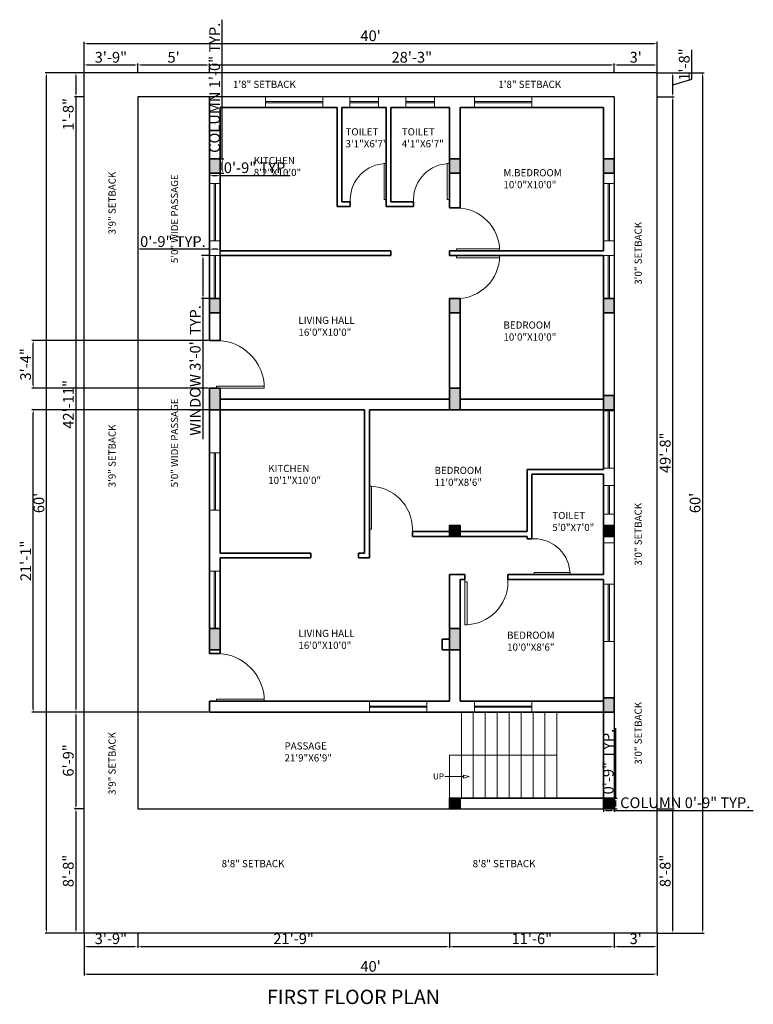
# Model space of a CAD drawing. Units: inches. Extents: x 3321 to 5237, y 11 to 1752.
# Tile 3 of 43: x 3968 to 4582, y 11 to 835. Entities that reach past the tile are written whole.
import ezdxf

# ---------------------------------------------------------------- set-up
doc = ezdxf.new("R2010")
doc.units = ezdxf.units.IN
for name, color, linetype, lineweight in [('A-ANNO-DIMS', 2, 'Continuous', 18), ('A-ANNO-SYMB', 7, 'Continuous', 18), ('A-ANNO-TEXT', 7, 'Continuous', 18), ('A-ANNO-TITL', 7, 'Continuous', 25), ('A-AREA-IDEN', 7, 'Continuous', 18), ('A-COLS', 1, 'Continuous', 35), ('A-DOOR', 4, 'Continuous', 18), ('A-FLOR-EDGE', 7, 'Continuous', 25), ('A-FLOR-STRS', 7, 'Continuous', 18), ('A-GLAZ', 5, 'Continuous', 18), ('A-WALL', 7, 'Continuous', 35), ('C-PROP', 7, 'Continuous', 30)]:
    doc.layers.add(name, color=color, linetype=linetype, lineweight=lineweight)
doc.styles.get("Standard").update_dxf_attribs({"font": 'arial.ttf'})
doc.dimstyles.new('ISO-25', dxfattribs={"dimtxt": 9, "dimasz": 2.5, "dimexe": 1.25, "dimexo": 0.625, "dimtad": 1, "dimdec": 1, "dimlunit": 3, "dimtxsty": 'Standard', "dimcen": 2.5, "dimclrd": 4, "dimclre": 4, "dimclrt": 256, "dimadec": 0, "dimazin": 0, "dimtfac": 1, "dimtdec": 1, "dimtmove": 0, "dimatfit": 3, "dimfxl": 1, "dimarcsym": 0})

# ---------------------------------------------------------------- blocks, each defined once
blk = doc.blocks.new('*U2')
for p, q in [((0, 0), (0, -6)), ((-40, 0), (-40, -6))]:
    blk.add_line(p, q)
blk.add_lwpolyline([(0, 0), (0, 40), (-1.75, 40), (-1.75, 0)], close=True)
blk.add_arc((0, 0), 40, 90, 180)
blk = doc.blocks.new('*U4')
for p, q in [((0, 0), (0, -6)), ((-36, 0), (-36, -6))]:
    blk.add_line(p, q)
blk.add_lwpolyline([(0, 0), (0, 36), (-1.75, 36), (-1.75, 0)], close=True)
blk.add_arc((0, 0), 36, 90, 180)
blk = doc.blocks.new('*U5')
for p, q in [((0, 0), (0, -6)), ((-30, 0), (-30, -6))]:
    blk.add_line(p, q)
blk.add_lwpolyline([(0, 0), (0, 30), (-1.75, 30), (-1.75, 0)], close=True)
blk.add_arc((0, 0), 30, 90, 180)
blk = doc.blocks.new('*U9')
for p, q in [((-36, 0), (-36, 6)), ((0, 0), (0, 6))]:
    blk.add_line(p, q)
blk.add_lwpolyline([(0, 0), (0, -36), (-1.75, -36), (-1.75, 0)], close=True)
blk.add_arc((0, 0), 36, 180, 270)
blk = doc.blocks.new('*D100')
at = {"layer": 'A-ANNO-DIMS', "color": 0, "lineweight": -2, "transparency": 16777216}
for p, q in [((4021.39, 791.23), (4021.39, 798.5)), ((4023.89, 797.25), (4063.89, 797.25)), ((4066.39, 791.23), (4066.39, 798.5))]:
    blk.add_line(p, q, dxfattribs=at)
at = {"layer": 'A-ANNO-DIMS', "color": 0, "transparency": 16777216}
for points in [[(4023.89, 797.66), (4023.89, 796.83), (4021.39, 797.25)], [(4063.89, 797.66), (4063.89, 796.83), (4066.39, 797.25)]]:
    blk.add_solid(points, dxfattribs=at)
at = {"layer": 'Defpoints', "color": 0, "transparency": 16777216}
for p in [(4066.39, 797.25), (4021.39, 790.61), (4066.39, 790.61)]:
    blk.add_point(p, dxfattribs=at)
at = {"layer": 'A-ANNO-DIMS', "color": 0, "transparency": 16777216, "insert": (4043.89, 802.47), "char_height": 9, "attachment_point": 5}
blk.add_mtext('3\'-9"', dxfattribs=at)
blk = doc.blocks.new('*D88')
at = {"layer": 'A-ANNO-DIMS', "color": 0, "lineweight": -2, "transparency": 16777216}
for p, q in [((4066.39, 791.23), (4066.39, 798.5)), ((4068.89, 797.25), (4123.89, 797.25)), ((4126.39, 791.23), (4126.39, 798.5))]:
    blk.add_line(p, q, dxfattribs=at)
at = {"layer": 'A-ANNO-DIMS', "color": 0, "transparency": 16777216}
for points in [[(4068.89, 797.66), (4068.89, 796.83), (4066.39, 797.25)], [(4123.89, 797.66), (4123.89, 796.83), (4126.39, 797.25)]]:
    blk.add_solid(points, dxfattribs=at)
at = {"layer": 'Defpoints', "color": 0, "transparency": 16777216}
for p in [(4126.39, 797.25), (4066.39, 790.61), (4126.39, 790.61)]:
    blk.add_point(p, dxfattribs=at)
at = {"layer": 'A-ANNO-DIMS', "color": 0, "transparency": 16777216, "insert": (4096.39, 802.45), "char_height": 9, "attachment_point": 5}
blk.add_mtext("5'", dxfattribs=at)
blk = doc.blocks.new('*D89')
at = {"layer": 'A-ANNO-DIMS', "color": 0, "lineweight": -2, "transparency": 16777216}
for p, q in [((4126.39, 791.23), (4126.39, 798.5)), ((4128.89, 797.25), (4462.89, 797.25)), ((4465.39, 791.23), (4465.39, 798.5))]:
    blk.add_line(p, q, dxfattribs=at)
at = {"layer": 'A-ANNO-DIMS', "color": 0, "transparency": 16777216}
for points in [[(4128.89, 797.66), (4128.89, 796.83), (4126.39, 797.25)], [(4462.89, 797.66), (4462.89, 796.83), (4465.39, 797.25)]]:
    blk.add_solid(points, dxfattribs=at)
at = {"layer": 'Defpoints', "color": 0, "transparency": 16777216}
for p in [(4465.39, 797.25), (4126.39, 790.61), (4465.39, 790.61)]:
    blk.add_point(p, dxfattribs=at)
at = {"layer": 'A-ANNO-DIMS', "color": 0, "transparency": 16777216, "insert": (4295.89, 802.47), "char_height": 9, "attachment_point": 5}
blk.add_mtext('28\'-3"', dxfattribs=at)
blk = doc.blocks.new('*D98')
at = {"layer": 'A-ANNO-DIMS', "color": 0, "lineweight": -2, "transparency": 16777216}
for p, q in [((4465.39, 791.23), (4465.39, 798.5)), ((4467.89, 797.25), (4498.89, 797.25)), ((4501.39, 791.23), (4501.39, 798.5))]:
    blk.add_line(p, q, dxfattribs=at)
at = {"layer": 'A-ANNO-DIMS', "color": 0, "transparency": 16777216}
for points in [[(4467.89, 797.66), (4467.89, 796.83), (4465.39, 797.25)], [(4498.89, 797.66), (4498.89, 796.83), (4501.39, 797.25)]]:
    blk.add_solid(points, dxfattribs=at)
at = {"layer": 'Defpoints', "color": 0, "transparency": 16777216}
for p in [(4501.39, 797.25), (4465.39, 790.61), (4501.39, 790.61)]:
    blk.add_point(p, dxfattribs=at)
at = {"layer": 'A-ANNO-DIMS', "color": 0, "transparency": 16777216, "insert": (4483.39, 802.47), "char_height": 9, "attachment_point": 5}
blk.add_mtext("3'", dxfattribs=at)
blk = doc.blocks.new('*D90')
at = {"layer": 'A-ANNO-DIMS', "color": 0, "lineweight": -2, "transparency": 16777216}
for p, q in [((4020.76, 790.61), (4013.34, 790.61)), ((4014.59, 788.11), (4014.59, 773.11)), ((4020.76, 770.61), (4013.34, 770.61)), ((4014.59, 770.61), (4014.59, 743.78))]:
    blk.add_line(p, q, dxfattribs=at)
at = {"layer": 'A-ANNO-DIMS', "color": 0, "transparency": 16777216}
for points in [[(4014.17, 788.11), (4015, 788.11), (4014.59, 790.61)], [(4014.17, 773.11), (4015, 773.11), (4014.59, 770.61)]]:
    blk.add_solid(points, dxfattribs=at)
at = {"layer": 'Defpoints', "color": 0, "transparency": 16777216}
for p in [(4021.39, 790.61), (4014.59, 770.61), (4021.39, 770.61)]:
    blk.add_point(p, dxfattribs=at)
at = {"layer": 'A-ANNO-DIMS', "color": 0, "transparency": 16777216, "insert": (4009.37, 755.94), "char_height": 9, "attachment_point": 5, "rotation": 90}
blk.add_mtext('1\'-8"', dxfattribs=at)
blk = doc.blocks.new('*D91')
at = {"layer": 'A-ANNO-DIMS', "color": 0, "lineweight": -2, "transparency": 16777216}
for p, q in [((4020.76, 770.61), (4013.34, 770.61)), ((4014.59, 768.11), (4014.59, 258.11)), ((4020.76, 255.61), (4013.34, 255.61))]:
    blk.add_line(p, q, dxfattribs=at)
at = {"layer": 'A-ANNO-DIMS', "color": 0, "transparency": 16777216}
for points in [[(4014.17, 768.11), (4015, 768.11), (4014.59, 770.61)], [(4014.17, 258.11), (4015, 258.11), (4014.59, 255.61)]]:
    blk.add_solid(points, dxfattribs=at)
at = {"layer": 'Defpoints', "color": 0, "transparency": 16777216}
for p in [(4021.39, 770.61), (4014.59, 255.61), (4021.39, 255.61)]:
    blk.add_point(p, dxfattribs=at)
at = {"layer": 'A-ANNO-DIMS', "color": 0, "transparency": 16777216, "insert": (4009.44, 513.11), "char_height": 9, "attachment_point": 5, "rotation": 90}
blk.add_mtext('42\'-11"', dxfattribs=at)
blk = doc.blocks.new('*D92')
at = {"layer": 'A-ANNO-DIMS', "color": 0, "lineweight": -2, "transparency": 16777216}
for p, q in [((4020.76, 255.61), (4013.34, 255.61)), ((4014.59, 253.11), (4014.59, 177.11)), ((4020.76, 174.61), (4013.34, 174.61))]:
    blk.add_line(p, q, dxfattribs=at)
at = {"layer": 'A-ANNO-DIMS', "color": 0, "transparency": 16777216}
for points in [[(4014.17, 253.11), (4015, 253.11), (4014.59, 255.61)], [(4014.17, 177.11), (4015, 177.11), (4014.59, 174.61)]]:
    blk.add_solid(points, dxfattribs=at)
at = {"layer": 'Defpoints', "color": 0, "transparency": 16777216}
for p in [(4021.39, 255.61), (4014.59, 174.61), (4021.39, 174.61)]:
    blk.add_point(p, dxfattribs=at)
at = {"layer": 'A-ANNO-DIMS', "color": 0, "transparency": 16777216, "insert": (4009.37, 215.11), "char_height": 9, "attachment_point": 5, "rotation": 90}
blk.add_mtext('6\'-9"', dxfattribs=at)
blk = doc.blocks.new('*D99')
at = {"layer": 'A-ANNO-DIMS', "color": 0, "lineweight": -2, "transparency": 16777216}
for p, q in [((4020.76, 174.61), (4013.34, 174.61)), ((4014.59, 172.11), (4014.59, 73.11)), ((4020.76, 70.61), (4013.34, 70.61))]:
    blk.add_line(p, q, dxfattribs=at)
at = {"layer": 'A-ANNO-DIMS', "color": 0, "transparency": 16777216}
for points in [[(4014.17, 172.11), (4015, 172.11), (4014.59, 174.61)], [(4014.17, 73.11), (4015, 73.11), (4014.59, 70.61)]]:
    blk.add_solid(points, dxfattribs=at)
at = {"layer": 'Defpoints', "color": 0, "transparency": 16777216}
for p in [(4021.39, 174.61), (4014.59, 70.61), (4021.39, 70.61)]:
    blk.add_point(p, dxfattribs=at)
at = {"layer": 'A-ANNO-DIMS', "color": 0, "transparency": 16777216, "insert": (4009.37, 122.61), "char_height": 9, "attachment_point": 5, "rotation": 90}
blk.add_mtext('8\'-8"', dxfattribs=at)
blk = doc.blocks.new('*D93')
at = {"layer": 'A-ANNO-DIMS', "color": 0, "lineweight": -2, "transparency": 16777216}
for p, q in [((4021.39, 69.98), (4021.39, 58.26)), ((4066.39, 69.98), (4066.39, 58.26)), ((4023.89, 59.51), (4063.89, 59.51))]:
    blk.add_line(p, q, dxfattribs=at)
at = {"layer": 'A-ANNO-DIMS', "color": 0, "transparency": 16777216}
for points in [[(4023.89, 59.93), (4023.89, 59.09), (4021.39, 59.51)], [(4063.89, 59.93), (4063.89, 59.09), (4066.39, 59.51)]]:
    blk.add_solid(points, dxfattribs=at)
at = {"layer": 'Defpoints', "color": 0, "transparency": 16777216}
for p in [(4021.39, 70.61), (4066.39, 70.61), (4066.39, 59.51)]:
    blk.add_point(p, dxfattribs=at)
at = {"layer": 'A-ANNO-DIMS', "color": 0, "transparency": 16777216, "insert": (4043.89, 64.73), "char_height": 9, "attachment_point": 5}
blk.add_mtext('3\'-9"', dxfattribs=at)
blk = doc.blocks.new('*D94')
at = {"layer": 'A-ANNO-DIMS', "color": 0, "lineweight": -2, "transparency": 16777216}
for p, q in [((4066.39, 69.98), (4066.39, 58.26)), ((4327.39, 69.98), (4327.39, 58.26)), ((4068.89, 59.51), (4324.89, 59.51))]:
    blk.add_line(p, q, dxfattribs=at)
at = {"layer": 'A-ANNO-DIMS', "color": 0, "transparency": 16777216}
for points in [[(4068.89, 59.93), (4068.89, 59.09), (4066.39, 59.51)], [(4324.89, 59.93), (4324.89, 59.09), (4327.39, 59.51)]]:
    blk.add_solid(points, dxfattribs=at)
at = {"layer": 'Defpoints', "color": 0, "transparency": 16777216}
for p in [(4066.39, 70.61), (4327.39, 70.61), (4327.39, 59.51)]:
    blk.add_point(p, dxfattribs=at)
at = {"layer": 'A-ANNO-DIMS', "color": 0, "transparency": 16777216, "insert": (4196.89, 64.73), "char_height": 9, "attachment_point": 5}
blk.add_mtext('21\'-9"', dxfattribs=at)
blk = doc.blocks.new('*D95')
at = {"layer": 'A-ANNO-DIMS', "color": 0, "lineweight": -2, "transparency": 16777216}
for p, q in [((4327.39, 69.98), (4327.39, 58.26)), ((4465.39, 69.98), (4465.39, 58.26)), ((4329.89, 59.51), (4462.89, 59.51))]:
    blk.add_line(p, q, dxfattribs=at)
at = {"layer": 'A-ANNO-DIMS', "color": 0, "transparency": 16777216}
for points in [[(4329.89, 59.93), (4329.89, 59.09), (4327.39, 59.51)], [(4462.89, 59.93), (4462.89, 59.09), (4465.39, 59.51)]]:
    blk.add_solid(points, dxfattribs=at)
at = {"layer": 'Defpoints', "color": 0, "transparency": 16777216}
for p in [(4327.39, 70.61), (4465.39, 70.61), (4465.39, 59.51)]:
    blk.add_point(p, dxfattribs=at)
at = {"layer": 'A-ANNO-DIMS', "color": 0, "transparency": 16777216, "insert": (4396.39, 64.73), "char_height": 9, "attachment_point": 5}
blk.add_mtext('11\'-6"', dxfattribs=at)
blk = doc.blocks.new('*D96')
at = {"layer": 'A-ANNO-DIMS', "color": 0, "lineweight": -2, "transparency": 16777216}
for p, q in [((4465.39, 69.98), (4465.39, 58.26)), ((4501.39, 69.98), (4501.39, 58.26)), ((4467.89, 59.51), (4498.89, 59.51))]:
    blk.add_line(p, q, dxfattribs=at)
at = {"layer": 'A-ANNO-DIMS', "color": 0, "transparency": 16777216}
for points in [[(4467.89, 59.93), (4467.89, 59.09), (4465.39, 59.51)], [(4498.89, 59.93), (4498.89, 59.09), (4501.39, 59.51)]]:
    blk.add_solid(points, dxfattribs=at)
at = {"layer": 'Defpoints', "color": 0, "transparency": 16777216}
for p in [(4465.39, 70.61), (4501.39, 70.61), (4501.39, 59.51)]:
    blk.add_point(p, dxfattribs=at)
at = {"layer": 'A-ANNO-DIMS', "color": 0, "transparency": 16777216, "insert": (4483.39, 64.73), "char_height": 9, "attachment_point": 5}
blk.add_mtext("3'", dxfattribs=at)
blk = doc.blocks.new('*D97')
at = {"layer": 'A-ANNO-DIMS', "color": 0, "lineweight": -2, "transparency": 16777216}
for p, q in [((4502.01, 174.61), (4515.69, 174.61)), ((4514.44, 73.11), (4514.44, 172.11)), ((4502.01, 70.61), (4515.69, 70.61))]:
    blk.add_line(p, q, dxfattribs=at)
at = {"layer": 'A-ANNO-DIMS', "color": 0, "transparency": 16777216}
for points in [[(4514.03, 172.11), (4514.86, 172.11), (4514.44, 174.61)], [(4514.03, 73.11), (4514.86, 73.11), (4514.44, 70.61)]]:
    blk.add_solid(points, dxfattribs=at)
at = {"layer": 'Defpoints', "color": 0, "transparency": 16777216}
for p in [(4501.39, 174.61), (4514.44, 174.61), (4501.39, 70.61)]:
    blk.add_point(p, dxfattribs=at)
at = {"layer": 'A-ANNO-DIMS', "color": 0, "transparency": 16777216, "insert": (4509.22, 122.61), "char_height": 9, "attachment_point": 5, "rotation": 90}
blk.add_mtext('8\'-8"', dxfattribs=at)
blk = doc.blocks.new('*D86')
at = {"layer": 'A-ANNO-DIMS', "color": 0, "lineweight": -2, "transparency": 16777216}
for p, q in [((4502.01, 770.61), (4515.69, 770.61)), ((4514.44, 177.11), (4514.44, 768.11)), ((4502.01, 174.61), (4515.69, 174.61))]:
    blk.add_line(p, q, dxfattribs=at)
at = {"layer": 'A-ANNO-DIMS', "color": 0, "transparency": 16777216}
for points in [[(4514.03, 768.11), (4514.86, 768.11), (4514.44, 770.61)], [(4514.03, 177.11), (4514.86, 177.11), (4514.44, 174.61)]]:
    blk.add_solid(points, dxfattribs=at)
at = {"layer": 'Defpoints', "color": 0, "transparency": 16777216}
for p in [(4501.39, 770.61), (4514.44, 770.61), (4501.39, 174.61)]:
    blk.add_point(p, dxfattribs=at)
at = {"layer": 'A-ANNO-DIMS', "color": 0, "transparency": 16777216, "insert": (4509.22, 472.61), "char_height": 9, "attachment_point": 5, "rotation": 90}
blk.add_mtext('49\'-8"', dxfattribs=at)
blk = doc.blocks.new('*D87')
at = {"layer": 'A-ANNO-DIMS', "color": 0, "lineweight": -2, "transparency": 16777216}
for p, q in [((4530.42, 785.4), (4530.42, 809.73)), ((4502.01, 790.61), (4515.69, 790.61)), ((4514.44, 773.11), (4514.44, 788.11)), ((4514.44, 780.61), (4530.42, 785.4)), ((4502.01, 770.61), (4515.69, 770.61))]:
    blk.add_line(p, q, dxfattribs=at)
at = {"layer": 'A-ANNO-DIMS', "color": 0, "transparency": 16777216}
for points in [[(4514.03, 788.11), (4514.86, 788.11), (4514.44, 790.61)], [(4514.03, 773.11), (4514.86, 773.11), (4514.44, 770.61)]]:
    blk.add_solid(points, dxfattribs=at)
at = {"layer": 'Defpoints', "color": 0, "transparency": 16777216}
for p in [(4501.39, 790.61), (4514.44, 790.61), (4501.39, 770.61)]:
    blk.add_point(p, dxfattribs=at)
at = {"layer": 'A-ANNO-DIMS', "color": 0, "transparency": 16777216, "insert": (4525.2, 797.56), "char_height": 9, "attachment_point": 5, "rotation": 90}
blk.add_mtext('1\'-8"', dxfattribs=at)
blk = doc.blocks.new('*D101')
at = {"layer": 'A-ANNO-DIMS', "color": 0, "lineweight": -2, "transparency": 16777216}
for p, q in [((4021.39, 791.23), (4021.39, 816.49)), ((4501.39, 791.23), (4501.39, 816.49)), ((4023.89, 815.24), (4498.89, 815.24))]:
    blk.add_line(p, q, dxfattribs=at)
at = {"layer": 'A-ANNO-DIMS', "color": 0, "transparency": 16777216}
for points in [[(4023.89, 815.66), (4023.89, 814.82), (4021.39, 815.24)], [(4498.89, 815.66), (4498.89, 814.82), (4501.39, 815.24)]]:
    blk.add_solid(points, dxfattribs=at)
at = {"layer": 'Defpoints', "color": 0, "transparency": 16777216}
for p in [(4501.39, 815.24), (4021.39, 790.61), (4501.39, 790.61)]:
    blk.add_point(p, dxfattribs=at)
at = {"layer": 'A-ANNO-DIMS', "color": 0, "transparency": 16777216, "insert": (4261.39, 820.46), "char_height": 9, "attachment_point": 5}
blk.add_mtext("40'", dxfattribs=at)
blk = doc.blocks.new('*D102')
at = {"layer": 'A-ANNO-DIMS', "color": 0, "lineweight": -2, "transparency": 16777216}
for p, q in [((4502.01, 790.61), (4540.73, 790.61)), ((4539.48, 73.11), (4539.48, 788.11)), ((4502.01, 70.61), (4540.73, 70.61))]:
    blk.add_line(p, q, dxfattribs=at)
at = {"layer": 'A-ANNO-DIMS', "color": 0, "transparency": 16777216}
for points in [[(4539.06, 788.11), (4539.9, 788.11), (4539.48, 790.61)], [(4539.06, 73.11), (4539.9, 73.11), (4539.48, 70.61)]]:
    blk.add_solid(points, dxfattribs=at)
at = {"layer": 'Defpoints', "color": 0, "transparency": 16777216}
for p in [(4501.39, 790.61), (4539.48, 790.61), (4501.39, 70.61)]:
    blk.add_point(p, dxfattribs=at)
at = {"layer": 'A-ANNO-DIMS', "color": 0, "transparency": 16777216, "insert": (4534.26, 430.61), "char_height": 9, "attachment_point": 5, "rotation": 90}
blk.add_mtext("60'", dxfattribs=at)
blk = doc.blocks.new('*D103')
at = {"layer": 'A-ANNO-DIMS', "color": 0, "lineweight": -2, "transparency": 16777216}
for p, q in [((4020.76, 790.61), (3988.74, 790.61)), ((3989.99, 73.11), (3989.99, 788.11)), ((4020.76, 70.61), (3988.74, 70.61))]:
    blk.add_line(p, q, dxfattribs=at)
at = {"layer": 'A-ANNO-DIMS', "color": 0, "transparency": 16777216}
for points in [[(3989.57, 788.11), (3990.4, 788.11), (3989.99, 790.61)], [(3989.57, 73.11), (3990.4, 73.11), (3989.99, 70.61)]]:
    blk.add_solid(points, dxfattribs=at)
at = {"layer": 'Defpoints', "color": 0, "transparency": 16777216}
for p in [(3989.99, 790.61), (4021.39, 790.61), (4021.39, 70.61)]:
    blk.add_point(p, dxfattribs=at)
at = {"layer": 'A-ANNO-DIMS', "color": 0, "transparency": 16777216, "insert": (3984.77, 430.61), "char_height": 9, "attachment_point": 5, "rotation": 90}
blk.add_mtext("60'", dxfattribs=at)
blk = doc.blocks.new('*D104')
at = {"layer": 'A-ANNO-DIMS', "color": 0, "lineweight": -2, "transparency": 16777216}
for p, q in [((4021.39, 69.98), (4021.39, 35.11)), ((4501.39, 69.98), (4501.39, 35.11)), ((4023.89, 36.36), (4498.89, 36.36))]:
    blk.add_line(p, q, dxfattribs=at)
at = {"layer": 'A-ANNO-DIMS', "color": 0, "transparency": 16777216}
for points in [[(4023.89, 36.78), (4023.89, 35.95), (4021.39, 36.36)], [(4498.89, 36.78), (4498.89, 35.95), (4501.39, 36.36)]]:
    blk.add_solid(points, dxfattribs=at)
at = {"layer": 'Defpoints', "color": 0, "transparency": 16777216}
for p in [(4021.39, 70.61), (4501.39, 70.61), (4501.39, 36.36)]:
    blk.add_point(p, dxfattribs=at)
at = {"layer": 'A-ANNO-DIMS', "color": 0, "transparency": 16777216, "insert": (4261.39, 41.58), "char_height": 9, "attachment_point": 5}
blk.add_mtext("40'", dxfattribs=at)
blk = doc.blocks.new('COL-9X18-IN')
h = blk.add_hatch(color=256)
h.dxf.hatch_style = 1
h.paths.add_polyline_path([(9, 18), (0, 18), (0, 0), (9, 0)])
blk.add_lwpolyline([(0, 0), (9, 0), (9, 18), (0, 18)], close=True)
blk = doc.blocks.new('COL-9X12-BASE-PLAN')
h = blk.add_hatch(color=256)
h.dxf.hatch_style = 1
h.paths.add_polyline_path([(0, 0), (9, 0), (9, 12), (0, 12)])
blk.add_lwpolyline([(0, 0), (9, 0), (9, 12), (0, 12)], close=True)
blk = doc.blocks.new('COL-9X9-BASE-PLAN')
h = blk.add_hatch(color=256)
h.dxf.hatch_style = 1
h.paths.add_polyline_path([(0, 0), (9, 0), (9, 9), (0, 9)])
blk.add_lwpolyline([(0, 0), (9, 0), (9, 9), (0, 9)], close=True)
blk = doc.blocks.new('WIN-48IN-9IN-WALL')
for p, q in [((0, 0), (0, 9)), ((48, 0), (48, 9)), ((0, 5), (48, 5)), ((0, 4), (48, 4))]:
    blk.add_line(p, q)
blk = doc.blocks.new('WIN-24IN-9IN-WALL')
for p, q in [((9, 24), (0, 24)), ((4, 24), (4, 0)), ((5, 24), (5, 0)), ((9, 0), (0, 0))]:
    blk.add_line(p, q)
blk = doc.blocks.new('WIN-36IN-9IN-WALL')
for p, q in [((9, 36), (0, 36)), ((4, 36), (4, 0)), ((5, 36), (5, 0)), ((9, 0), (0, 0))]:
    blk.add_line(p, q)
blk = doc.blocks.new('STAIR-RETURN-72IN')
for p, q in [((10, 72), (10, 0)), ((20, 72), (20, 0)), ((30, 72), (30, 0)), ((40, 72), (40, 0)), ((50, 72), (50, 0)), ((60, 72), (60, 0)), ((70, 72), (70, 0)), ((80, 72), (80, 0)), ((90, 72), (90, 0)), ((90, 36), (0, 36)), ((0, 36), (0, 0))]:
    blk.add_line(p, q)
blk = doc.blocks.new('STAIR-DIRECTION-ARROW')
blk.add_line((0, 1.22), (15.43, 1.22))
blk.add_lwpolyline([(20.27, 1.22), (15.43, 2.43), (15.43, 0)], close=True)
blk = doc.blocks.new('PROPERTY-40X60FT')
for p, q in [((0, 720), (480, 720)), ((0, 720), (0, 0)), ((480, 720), (480, 0)), ((0, 0), (480, 0))]:
    blk.add_line(p, q)
blk = doc.blocks.new('*D169')
at = {"layer": 'A-ANNO-DIMS', "color": 4, "lineweight": -2, "transparency": 16777216}
for p, q in [((4125.76, 637.61), (4119.74, 637.61)), ((4120.99, 635.11), (4120.99, 604.11)), ((4125.76, 601.61), (4119.74, 601.61)), ((4120.99, 601.61), (4120.99, 483.97))]:
    blk.add_line(p, q, dxfattribs=at)
at = {"layer": 'A-ANNO-DIMS', "color": 4, "transparency": 16777216}
for points in [[(4120.57, 635.11), (4121.4, 635.11), (4120.99, 637.61)], [(4120.57, 604.11), (4121.4, 604.11), (4120.99, 601.61)]]:
    blk.add_solid(points, dxfattribs=at)
at = {"layer": 'Defpoints', "color": 0, "transparency": 16777216}
for p in [(4126.39, 637.61), (4120.99, 601.61), (4126.39, 601.61)]:
    blk.add_point(p, dxfattribs=at)
at = {"layer": 'A-ANNO-DIMS', "transparency": 16777216, "insert": (4115.7, 541.54), "char_height": 9, "attachment_point": 5, "rotation": 90}
blk.add_mtext('WINDOW 3\'-0" TYP.', dxfattribs=at)
blk = doc.blocks.new('*D170')
at = {"layer": 'A-ANNO-DIMS', "color": 4, "lineweight": -2, "transparency": 16777216}
for p, q in [((4126.39, 643.01), (4067.78, 643.01)), ((4126.39, 638.23), (4126.39, 644.26)), ((4132.89, 643.01), (4128.89, 643.01)), ((4135.39, 638.23), (4135.39, 644.26))]:
    blk.add_line(p, q, dxfattribs=at)
at = {"layer": 'A-ANNO-DIMS', "color": 4, "transparency": 16777216}
for points in [[(4128.89, 643.42), (4128.89, 642.59), (4126.39, 643.01)], [(4132.89, 643.42), (4132.89, 642.59), (4135.39, 643.01)]]:
    blk.add_solid(points, dxfattribs=at)
at = {"layer": 'Defpoints', "color": 0, "transparency": 16777216}
for p in [(4126.39, 643.01), (4126.39, 637.61), (4135.39, 637.61)]:
    blk.add_point(p, dxfattribs=at)
at = {"layer": 'A-ANNO-DIMS', "transparency": 16777216, "insert": (4095.83, 648.23), "char_height": 9, "attachment_point": 5}
blk.add_mtext('0\'-9" TYP.', dxfattribs=at)
blk = doc.blocks.new('*D185')
at = {"layer": 'A-ANNO-DIMS', "color": 4, "lineweight": -2, "transparency": 16777216}
for p, q in [((4137.19, 718.61), (4137.19, 835.09)), ((4136.01, 718.61), (4138.44, 718.61)), ((4137.19, 709.11), (4137.19, 716.11)), ((4136.01, 706.61), (4138.44, 706.61))]:
    blk.add_line(p, q, dxfattribs=at)
at = {"layer": 'A-ANNO-DIMS', "color": 4, "transparency": 16777216}
for points in [[(4136.77, 716.11), (4137.6, 716.11), (4137.19, 718.61)], [(4136.77, 709.11), (4137.6, 709.11), (4137.19, 706.61)]]:
    blk.add_solid(points, dxfattribs=at)
at = {"layer": 'Defpoints', "color": 0, "transparency": 16777216}
for p in [(4135.39, 718.61), (4137.19, 718.61), (4135.39, 706.61)]:
    blk.add_point(p, dxfattribs=at)
at = {"layer": 'A-ANNO-DIMS', "transparency": 16777216, "insert": (4131.9, 778.1), "char_height": 9, "attachment_point": 5, "rotation": 90}
blk.add_mtext('COLUMN 1\'-0" TYP.', dxfattribs=at)
blk = doc.blocks.new('*D186')
at = {"layer": 'A-ANNO-DIMS', "color": 4, "lineweight": -2, "transparency": 16777216}
for p, q in [((4126.39, 705.98), (4126.39, 703.56)), ((4128.89, 704.81), (4132.89, 704.81)), ((4135.39, 705.98), (4135.39, 703.56)), ((4135.39, 704.81), (4194, 704.81))]:
    blk.add_line(p, q, dxfattribs=at)
at = {"layer": 'A-ANNO-DIMS', "color": 4, "transparency": 16777216}
for points in [[(4128.89, 705.22), (4128.89, 704.39), (4126.39, 704.81)], [(4132.89, 705.22), (4132.89, 704.39), (4135.39, 704.81)]]:
    blk.add_solid(points, dxfattribs=at)
at = {"layer": 'Defpoints', "color": 0, "transparency": 16777216}
for p in [(4126.39, 706.61), (4135.39, 706.61), (4135.39, 704.81)]:
    blk.add_point(p, dxfattribs=at)
at = {"layer": 'A-ANNO-DIMS', "transparency": 16777216, "insert": (4165.94, 710.03), "char_height": 9, "attachment_point": 5}
blk.add_mtext('0\'-9" TYP.', dxfattribs=at)
blk = doc.blocks.new('*D187')
at = {"layer": 'A-ANNO-DIMS', "color": 4, "lineweight": -2, "transparency": 16777216}
for p, q in [((4456.39, 173.98), (4456.39, 172.01)), ((4458.89, 173.26), (4462.89, 173.26)), ((4465.39, 173.98), (4465.39, 172.01)), ((4465.39, 173.26), (4581.87, 173.26))]:
    blk.add_line(p, q, dxfattribs=at)
at = {"layer": 'A-ANNO-DIMS', "color": 4, "transparency": 16777216}
for points in [[(4458.89, 173.67), (4458.89, 172.84), (4456.39, 173.26)], [(4462.89, 173.67), (4462.89, 172.84), (4465.39, 173.26)]]:
    blk.add_solid(points, dxfattribs=at)
at = {"layer": 'Defpoints', "color": 0, "transparency": 16777216}
for p in [(4456.39, 174.61), (4465.39, 174.61), (4465.39, 173.26)]:
    blk.add_point(p, dxfattribs=at)
at = {"layer": 'A-ANNO-DIMS', "transparency": 16777216, "insert": (4524.88, 178.54), "char_height": 9, "attachment_point": 5}
blk.add_mtext('COLUMN 0\'-9" TYP.', dxfattribs=at)
blk = doc.blocks.new('*D188')
at = {"layer": 'A-ANNO-DIMS', "color": 4, "lineweight": -2, "transparency": 16777216}
for p, q in [((4466.74, 183.61), (4466.74, 242.22)), ((4466.01, 183.61), (4467.99, 183.61)), ((4466.01, 174.61), (4467.99, 174.61)), ((4466.74, 177.11), (4466.74, 181.11))]:
    blk.add_line(p, q, dxfattribs=at)
at = {"layer": 'A-ANNO-DIMS', "color": 4, "transparency": 16777216}
for points in [[(4466.32, 181.11), (4467.15, 181.11), (4466.74, 183.61)], [(4466.32, 177.11), (4467.15, 177.11), (4466.74, 174.61)]]:
    blk.add_solid(points, dxfattribs=at)
at = {"layer": 'Defpoints', "color": 0, "transparency": 16777216}
for p in [(4465.39, 183.61), (4466.74, 183.61), (4465.39, 174.61)]:
    blk.add_point(p, dxfattribs=at)
at = {"layer": 'A-ANNO-DIMS', "transparency": 16777216, "insert": (4461.52, 214.16), "char_height": 9, "attachment_point": 5, "rotation": 90}
blk.add_mtext('0\'-9" TYP.', dxfattribs=at)
blk = doc.blocks.new('*D225')
at = {"layer": 'A-ANNO-DIMS', "color": 4, "lineweight": -2, "transparency": 16777216}
for p, q in [((4125.76, 508.61), (3977.64, 508.61)), ((3978.89, 258.11), (3978.89, 506.11)), ((4125.76, 255.61), (3977.64, 255.61))]:
    blk.add_line(p, q, dxfattribs=at)
at = {"layer": 'A-ANNO-DIMS', "color": 4, "transparency": 16777216}
for points in [[(3978.47, 506.11), (3979.3, 506.11), (3978.89, 508.61)], [(3978.47, 258.11), (3979.3, 258.11), (3978.89, 255.61)]]:
    blk.add_solid(points, dxfattribs=at)
at = {"layer": 'Defpoints', "color": 0, "transparency": 16777216}
for p in [(3978.89, 508.61), (4126.39, 508.61), (4126.39, 255.61)]:
    blk.add_point(p, dxfattribs=at)
at = {"layer": 'A-ANNO-DIMS', "transparency": 16777216, "insert": (3973.74, 382.11), "char_height": 9, "attachment_point": 5, "rotation": 90}
blk.add_mtext('21\'-1"', dxfattribs=at)
blk = doc.blocks.new('*D226')
at = {"layer": 'A-ANNO-DIMS', "color": 4, "lineweight": -2, "transparency": 16777216}
for p, q in [((4125.76, 566.61), (3977.64, 566.61)), ((3978.89, 529.11), (3978.89, 564.11)), ((4125.76, 526.61), (3977.64, 526.61))]:
    blk.add_line(p, q, dxfattribs=at)
at = {"layer": 'A-ANNO-DIMS', "color": 4, "transparency": 16777216}
for points in [[(3978.47, 564.11), (3979.3, 564.11), (3978.89, 566.61)], [(3978.47, 529.11), (3979.3, 529.11), (3978.89, 526.61)]]:
    blk.add_solid(points, dxfattribs=at)
at = {"layer": 'Defpoints', "color": 0, "transparency": 16777216}
for p in [(3978.89, 566.61), (4126.39, 566.61), (4126.39, 526.61)]:
    blk.add_point(p, dxfattribs=at)
at = {"layer": 'A-ANNO-DIMS', "transparency": 16777216, "insert": (3973.66, 546.61), "char_height": 9, "attachment_point": 5, "rotation": 90}
blk.add_mtext('3\'-4"', dxfattribs=at)

msp = doc.modelspace()

# ---------------------------------------------------------------- linework, layer by layer
at = {"layer": 'A-FLOR-EDGE'}
for p, q in [((4066.39, 770.61), (4066.39, 174.61)), ((4465.39, 770.61), (4066.39, 770.61)), ((4465.39, 770.61), (4465.39, 174.61)), ((4066.39, 174.61), (4465.39, 174.61))]:
    msp.add_line(p, q, dxfattribs=at)
at = {"layer": 'A-GLAZ'}
msp.add_line((4465.39, 397.11), (4456.39, 397.11), dxfattribs=at)
at = {"layer": 'A-WALL'}
for p, q in [((4126.39, 770.61), (4126.39, 566.61)), ((4135.39, 761.61), (4135.39, 641.61)), ((4233.39, 761.61), (4135.39, 761.61)), ((4233.39, 761.61), (4233.39, 678.61)), ((4237.39, 761.61), (4237.39, 682.61)), ((4274.39, 761.61), (4237.39, 761.61)), ((4274.39, 761.61), (4274.39, 678.61)), ((4278.39, 761.61), (4278.39, 682.61)), ((4327.39, 761.61), (4278.39, 761.61)), ((4327.39, 761.61), (4327.39, 677.61)), ((4336.39, 761.61), (4336.39, 677.61)), ((4456.39, 761.61), (4336.39, 761.61)), ((4456.39, 761.61), (4456.39, 641.61)), ((4244.39, 678.61), (4233.39, 678.61)), ((4244.39, 682.61), (4237.39, 682.61)), ((4244.39, 682.61), (4244.39, 678.61)), ((4297.39, 678.61), (4274.39, 678.61)), ((4297.39, 682.61), (4278.39, 682.61)), ((4297.39, 682.61), (4297.39, 678.61)), ((4336.39, 677.61), (4327.39, 677.61)), ((4278.39, 641.61), (4135.39, 641.61)), ((4135.39, 637.61), (4135.39, 566.61)), ((4135.39, 637.61), (4278.39, 637.61)), ((4278.39, 641.61), (4278.39, 637.61)), ((4327.39, 641.61), (4327.39, 637.61)), ((4456.39, 641.61), (4327.39, 641.61)), ((4327.39, 637.61), (4456.39, 637.61)), ((4456.39, 637.61), (4456.39, 517.61)), ((4327.39, 601.61), (4327.39, 526.61)), ((4327.39, 601.61), (4336.39, 601.61)), ((4336.39, 601.61), (4336.39, 517.61)), ((4126.39, 566.61), (4135.39, 566.61)), ((4126.39, 526.61), (4126.39, 304.61)), ((4126.39, 526.61), (4135.39, 526.61)), ((4135.39, 526.61), (4135.39, 517.61)), ((4135.39, 517.61), (4327.39, 517.61)), ((4336.39, 517.61), (4456.39, 517.61)), ((4135.39, 508.61), (4135.39, 388.61)), ((4135.39, 508.61), (4256.39, 508.61)), ((4256.39, 508.61), (4256.39, 388.61)), ((4260.39, 508.61), (4260.39, 384.61)), ((4260.39, 508.61), (4327.39, 508.61)), ((4336.39, 508.61), (4456.39, 508.61)), ((4456.39, 508.61), (4456.39, 458.61)), ((4392.39, 458.61), (4392.39, 406.61)), ((4392.39, 458.61), (4456.39, 458.61)), ((4396.39, 454.61), (4396.39, 400.61)), ((4396.39, 454.61), (4456.39, 454.61)), ((4456.39, 454.61), (4456.39, 370.61)), ((4296.39, 406.61), (4296.39, 402.61)), ((4296.39, 406.61), (4392.39, 406.61)), ((4296.39, 402.61), (4392.39, 402.61)), ((4392.39, 402.61), (4392.39, 400.61)), ((4392.39, 400.61), (4396.39, 400.61)), ((4135.39, 388.61), (4211.39, 388.61)), ((4211.39, 388.61), (4211.39, 384.61)), ((4251.39, 388.61), (4251.39, 384.61)), ((4251.39, 388.61), (4256.39, 388.61)), ((4135.39, 384.61), (4135.39, 304.61)), ((4135.39, 384.61), (4211.39, 384.61)), ((4251.39, 384.61), (4260.39, 384.61)), ((4327.39, 370.61), (4327.39, 316.61)), ((4327.39, 370.61), (4340.39, 370.61)), ((4336.39, 366.61), (4336.39, 264.61)), ((4336.39, 366.61), (4340.39, 366.61)), ((4340.39, 370.61), (4340.39, 366.61)), ((4376.39, 370.61), (4376.39, 366.61)), ((4376.39, 370.61), (4456.39, 370.61)), ((4376.39, 366.61), (4456.39, 366.61)), ((4456.39, 366.61), (4456.39, 264.61)), ((4321.39, 316.61), (4327.39, 316.61)), ((4321.39, 316.61), (4321.39, 307.61)), ((4321.39, 307.61), (4327.39, 307.61)), ((4327.39, 307.61), (4327.39, 264.61)), ((4126.39, 304.61), (4135.39, 304.61)), ((4126.39, 264.61), (4126.39, 255.61)), ((4126.39, 264.61), (4327.39, 264.61)), ((4336.39, 264.61), (4456.39, 264.61)), ((4126.39, 255.61), (4456.39, 255.61)), ((4456.39, 255.61), (4456.39, 183.61)), ((4327.39, 183.61), (4327.39, 174.61)), ((4327.39, 183.61), (4456.39, 183.61))]:
    msp.add_line(p, q, dxfattribs=at)

# ---------------------------------------------------------------- block references
at = {"layer": 'A-ANNO-SYMB'}
msp.add_blockref('STAIR-DIRECTION-ARROW', (4323.66, 200.39), dxfattribs=at)
at = {"layer": 'A-COLS'}
for name, p in [('COL-9X12-BASE-PLAN', (4126.39, 706.61)), ('COL-9X12-BASE-PLAN', (4327.39, 706.61)), ('COL-9X12-BASE-PLAN', (4456.39, 706.61)), ('COL-9X12-BASE-PLAN', (4126.39, 589.61)), ('COL-9X12-BASE-PLAN', (4327.39, 589.61)), ('COL-9X12-BASE-PLAN', (4456.39, 589.61)), ('COL-9X12-BASE-PLAN', (4456.39, 508.61)), ('COL-9X9-BASE-PLAN', (4327.39, 402.61)), ('COL-9X9-BASE-PLAN', (4456.39, 402.61)), ('COL-9X12-BASE-PLAN', (4456.39, 255.61)), ('COL-9X9-BASE-PLAN', (4327.39, 174.61)), ('COL-9X9-BASE-PLAN', (4456.39, 174.61))]:
    msp.add_blockref(name, p, dxfattribs=at)
at = {"layer": 'A-COLS', "rotation": 180}
for p in [(4135.39, 526.61), (4336.39, 526.61), (4135.39, 325.61), (4336.39, 325.61)]:
    msp.add_blockref('COL-9X18-IN', p, dxfattribs=at)
at = {"layer": 'A-DOOR'}
for p in [(4274.39, 684.61), (4327.39, 684.61)]:
    msp.add_blockref('*U5', p, dxfattribs=at)
at = {"layer": 'A-DOOR', "rotation": 270}
for name, p in [('*U4', (4333.39, 641.61)), ('*U2', (4132.39, 526.61)), ('*U5', (4398.39, 370.61)), ('*U2', (4132.39, 264.61))]:
    msp.add_blockref(name, p, dxfattribs=at)
at = {"layer": 'A-DOOR', "xscale": -1, "rotation": 270}
msp.add_blockref('*U4', (4333.39, 637.61), dxfattribs=at)
at = {"layer": 'A-DOOR', "xscale": -1}
for name, p in [('*U4', (4260.39, 408.61)), ('*U9', (4340.39, 364.61))]:
    msp.add_blockref(name, p, dxfattribs=at)
at = {"layer": 'A-FLOR-STRS'}
msp.add_blockref('STAIR-RETURN-72IN', (4327.39, 183.61), dxfattribs=at)
at = {"layer": 'A-GLAZ'}
for name, p in [('WIN-48IN-9IN-WALL', (4173.36, 761.61)), ('WIN-48IN-9IN-WALL', (4348.36, 761.61)), ('WIN-24IN-9IN-WALL', (4456.39, 421.11)), ('WIN-48IN-9IN-WALL', (4260.39, 255.61)), ('WIN-48IN-9IN-WALL', (4348.39, 255.61))]:
    msp.add_blockref(name, p, dxfattribs=at)
for name, p, rotation in [('WIN-24IN-9IN-WALL', (4243.89, 770.61), 269.9999999999962), ('WIN-24IN-9IN-WALL', (4290.89, 770.61), 269.9999999999976), ('WIN-48IN-9IN-WALL', (4135.39, 650.11), 89.99999999999818), ('WIN-48IN-9IN-WALL', (4465.39, 650.11), 89.99999999999818), ('WIN-36IN-9IN-WALL', (4135.39, 637.61), 180), ('WIN-36IN-9IN-WALL', (4465.39, 637.61), 180), ('WIN-48IN-9IN-WALL', (4465.39, 459.61), 89.99999999999818), ('WIN-48IN-9IN-WALL', (4135.39, 424.61), 89.99999999999613), ('WIN-48IN-9IN-WALL', (4135.39, 325.61), 89.99999999999824), ('WIN-48IN-9IN-WALL', (4465.39, 314.61), 89.99999999999406)]:
    msp.add_blockref(name, p, dxfattribs=dict(at, rotation=rotation))
at = {"layer": 'C-PROP', "rotation": 180}
msp.add_blockref('PROPERTY-40X60FT', (4501.39, 790.61), dxfattribs=at)

# ---------------------------------------------------------------- texts
at = {"layer": 'A-ANNO-TEXT'}
msp.add_text('UP', height=5, dxfattribs=at).set_placement((4313.6, 199.21))
at = {"layer": 'A-ANNO-TEXT', "char_height": 6, "attachment_point": 1}
for s, insert in [('1\'8" SETBACK', (4146.15, 783.97)), ('1\'8" SETBACK', (4368.37, 783.97)), ('8\'8" SETBACK', (4136.66, 131.73)), ('8\'8" SETBACK', (4346.85, 131.73))]:
    msp.add_mtext_dynamic_manual_height_columns(s, width=97.3114, gutter_width=25, heights=[0], dxfattribs=dict(at, insert=insert))
at = {"layer": 'A-ANNO-TEXT', "char_height": 6, "attachment_point": 1, "rotation": 90}
for s, insert in [('3\'9" SETBACK', (4041.9, 655.29)), ('3\'0" SETBACK', (4482.45, 613.28)), ('3\'9" SETBACK', (4041.9, 443.71)), ('3\'0" SETBACK', (4482.45, 378.11)), ('3\'0" SETBACK', (4482.45, 211.53)), ('3\'9" SETBACK', (4041.9, 186.23))]:
    msp.add_mtext_dynamic_manual_height_columns(s, width=97.3114, gutter_width=25, heights=[0], dxfattribs=dict(at, insert=insert))
at = {"layer": 'A-ANNO-TITL', "insert": (4174.67, 23.21), "char_height": 12, "attachment_point": 1}
msp.add_mtext_dynamic_manual_height_columns('FIRST FLOOR PLAN', width=241.3793, gutter_width=25, heights=[0], dxfattribs=at)
at = {"layer": 'A-AREA-IDEN', "char_height": 6, "attachment_point": 1}
for s, insert in [('TOILET\\P3\'1"X6\'7"', (4240.4, 744.24)), ('TOILET\\P4\'1"X6\'7"', (4287.51, 744.24)), ('KITCHEN\\P8\'2"X10\'0"', (4163.54, 720.23)), ('M.BEDROOM\\P10\'0"X10\'0"', (4372.64, 710.01)), ('LIVING HALL\\P16\'0"X10\'0"', (4200.96, 586.5)), ('BEDROOM\\P10\'0"X10\'0"', (4372.64, 582.52)), ('KITCHEN\\P10\'1"X10\'0"', (4175.65, 462.52)), ('BEDROOM\\P11\'0"X8\'6"', (4314.91, 460.88)), ('TOILET\\P5\'0"X7\'0"', (4413.53, 423.12)), ('LIVING HALL\\P16\'0"X10\'0"', (4200.96, 324.44)), ('BEDROOM\\P10\'0"X8\'6"', (4375.68, 322.94)), ('PASSAGE\\P21\'9"X6\'9" ', (4189.31, 230.23))]:
    msp.add_mtext_dynamic_manual_height_columns(s, width=97.3114, gutter_width=25, heights=[0], dxfattribs=dict(at, insert=insert))
at = {"layer": 'A-AREA-IDEN', "char_height": 6, "attachment_point": 1, "rotation": 90}
for insert in [(4094.18, 631.35), (4094.18, 443.71)]:
    msp.add_mtext_dynamic_manual_height_columns('5\'0" WIDE PASSAGE', width=97.3114, gutter_width=25, heights=[0], dxfattribs=dict(at, insert=insert))

# ---------------------------------------------------------------- dimensions: what is measured, and where the dimension line sits
at = {"layer": 'A-ANNO-DIMS'}
for base, p1, p2, angle, text, picture, middle in [((4137.19, 718.61), (4135.39, 706.61), (4135.39, 718.61), 90, 'COLUMN <> TYP.', '*D185', (4131.9, 778.1)), ((4126.39, 643.01), (4135.39, 637.61), (4126.39, 637.61), 180, '<> TYP.', '*D170', (4095.83, 648.23)), ((4120.99, 601.61), (4126.39, 637.61), (4126.39, 601.61), 270, 'WINDOW <> TYP.', '*D169', (4115.7, 541.54)), ((4466.74, 183.61), (4465.39, 174.61), (4465.39, 183.61), 90, '<> TYP.', '*D188', (4461.52, 214.16))]:
    dim = msp.add_linear_dim(base=base, p1=p1, p2=p2, angle=angle, text=text, dimstyle='ISO-25', override={"dimdec": 1, "dimlfac": 1, "dimrnd": 0, "dimzin": 1, "dimdsep": 46, "dimlunit": 4, "dimfrac": 2}, dxfattribs=at)
    dim.commit()
    dim.dimension.update_dxf_attribs({"geometry": picture, "text_midpoint": middle})
for base, p1, p2, override, picture, middle in [((4501.39, 815.24), (4021.39, 790.61), (4501.39, 790.61), {"dimclrd": 0, "dimclre": 0, "dimclrt": 0}, '*D101', (4261.39, 820.46)), ((4066.39, 797.25), (4021.39, 790.61), (4066.39, 790.61), {"dimclrd": 0, "dimclre": 0, "dimclrt": 0}, '*D100', (4043.89, 802.47)), ((4126.39, 797.25), (4066.39, 790.61), (4126.39, 790.61), {"dimclrd": 0, "dimclre": 0, "dimclrt": 0, "dimtmove": 1}, '*D88', (4096.39, 802.45)), ((4465.39, 797.25), (4126.39, 790.61), (4465.39, 790.61), {"dimclrd": 0, "dimclre": 0, "dimclrt": 0, "dimtmove": 1}, '*D89', (4295.89, 802.47)), ((4501.39, 797.25), (4465.39, 790.61), (4501.39, 790.61), {"dimclrd": 0, "dimclre": 0, "dimclrt": 0, "dimtmove": 1}, '*D98', (4483.39, 802.47)), ((4066.39, 59.51), (4021.39, 70.61), (4066.39, 70.61), {"dimclrd": 0, "dimclre": 0, "dimclrt": 0}, '*D93', (4043.89, 64.73)), ((4501.39, 36.36), (4021.39, 70.61), (4501.39, 70.61), {"dimclrd": 0, "dimclre": 0, "dimclrt": 0}, '*D104', (4261.39, 41.58)), ((4327.39, 59.51), (4066.39, 70.61), (4327.39, 70.61), {"dimclrd": 0, "dimclre": 0, "dimclrt": 0, "dimtmove": 1}, '*D94', (4196.89, 64.73)), ((4465.39, 59.51), (4327.39, 70.61), (4465.39, 70.61), {"dimclrd": 0, "dimclre": 0, "dimclrt": 0, "dimtmove": 1}, '*D95', (4396.39, 64.73)), ((4501.39, 59.51), (4465.39, 70.61), (4501.39, 70.61), {"dimclrd": 0, "dimclre": 0, "dimclrt": 0, "dimtmove": 1}, '*D96', (4483.39, 64.73))]:
    dim = msp.add_linear_dim(base=base, p1=p1, p2=p2, dimstyle='ISO-25', override=override, dxfattribs=at)
    dim.commit()
    dim.dimension.update_dxf_attribs({"geometry": picture, "text_midpoint": middle})
for base, p1, p2, angle, override, picture, middle in [((4514.44, 790.61), (4501.39, 770.61), (4501.39, 790.61), 90, {"dimclrd": 0, "dimclre": 0, "dimclrt": 0, "dimtmove": 1}, '*D87', (4525.2, 786.03)), ((3989.99, 790.61), (4021.39, 70.61), (4021.39, 790.61), 270, {"dimclrd": 0, "dimclre": 0, "dimclrt": 0}, '*D103', (3984.77, 430.61)), ((4014.59, 770.61), (4021.39, 790.61), (4021.39, 770.61), 90, {"dimclrd": 0, "dimclre": 0, "dimclrt": 0}, '*D90', (4009.37, 755.94)), ((4539.48, 790.61), (4501.39, 70.61), (4501.39, 790.61), 270, {"dimclrd": 0, "dimclre": 0, "dimclrt": 0}, '*D102', (4534.26, 430.61)), ((4014.59, 255.61), (4021.39, 770.61), (4021.39, 255.61), 90, {"dimclrd": 0, "dimclre": 0, "dimclrt": 0, "dimtmove": 1}, '*D91', (4009.44, 513.11)), ((4514.44, 770.61), (4501.39, 174.61), (4501.39, 770.61), 90, {"dimclrd": 0, "dimclre": 0, "dimclrt": 0, "dimtmove": 1}, '*D86', (4509.22, 472.61)), ((3978.89, 566.61), (4126.39, 526.61), (4126.39, 566.61), 90, {"dimdec": 1, "dimlfac": 1, "dimrnd": 0, "dimzin": 1, "dimdsep": 46, "dimlunit": 4, "dimfrac": 2}, '*D226', (3973.66, 546.61)), ((3978.89, 508.61), (4126.39, 255.61), (4126.39, 508.61), 90, {"dimdec": 1, "dimlfac": 1, "dimrnd": 0, "dimzin": 1, "dimdsep": 46, "dimlunit": 4, "dimfrac": 2}, '*D225', (3973.74, 382.11)), ((4014.59, 174.61), (4021.39, 255.61), (4021.39, 174.61), 90, {"dimclrd": 0, "dimclre": 0, "dimclrt": 0, "dimtmove": 1}, '*D92', (4009.37, 215.11)), ((4014.59, 70.61), (4021.39, 174.61), (4021.39, 70.61), 90, {"dimclrd": 0, "dimclre": 0, "dimclrt": 0, "dimtmove": 1}, '*D99', (4009.37, 122.61)), ((4514.44, 174.61), (4501.39, 70.61), (4501.39, 174.61), 90, {"dimclrd": 0, "dimclre": 0, "dimclrt": 0}, '*D97', (4509.22, 122.61))]:
    dim = msp.add_linear_dim(base=base, p1=p1, p2=p2, angle=angle, dimstyle='ISO-25', override=override, dxfattribs=at)
    dim.commit()
    dim.dimension.update_dxf_attribs({"geometry": picture, "text_midpoint": middle})
for base, p1, p2, text, picture, middle in [((4135.39, 704.81), (4126.39, 706.61), (4135.39, 706.61), '<> TYP.', '*D186', (4165.94, 710.03)), ((4465.39, 173.26), (4456.39, 174.61), (4465.39, 174.61), 'COLUMN <> TYP.', '*D187', (4524.88, 178.54))]:
    dim = msp.add_linear_dim(base=base, p1=p1, p2=p2, text=text, dimstyle='ISO-25', override={"dimdec": 1, "dimlfac": 1, "dimrnd": 0, "dimzin": 1, "dimdsep": 46, "dimlunit": 4, "dimfrac": 2}, dxfattribs=at)
    dim.commit()
    dim.dimension.update_dxf_attribs({"geometry": picture, "text_midpoint": middle})

doc.saveas('drawing.dxf')
